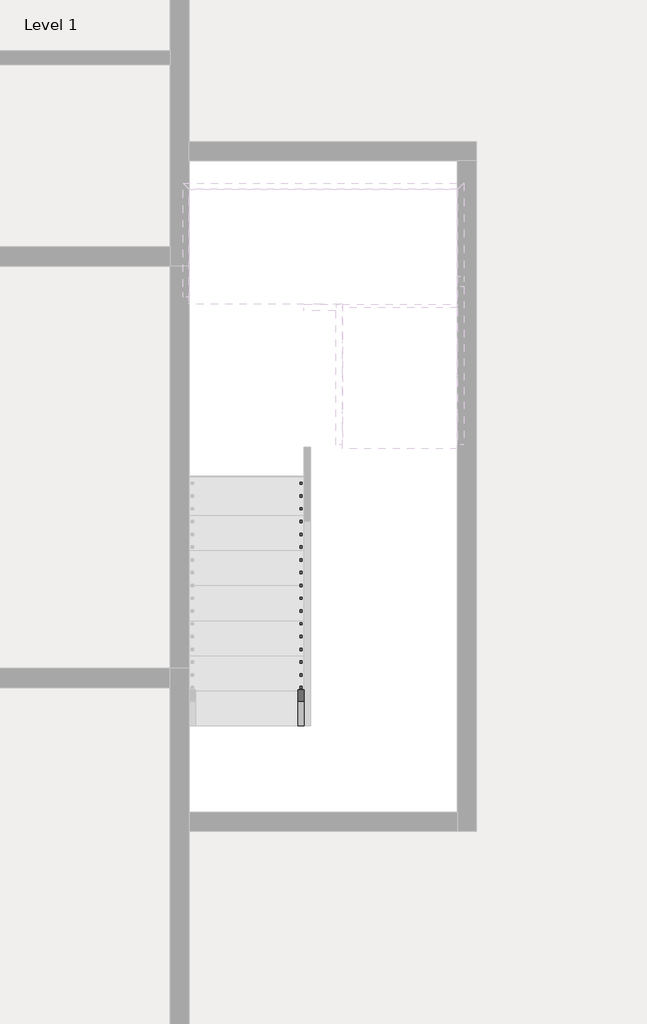
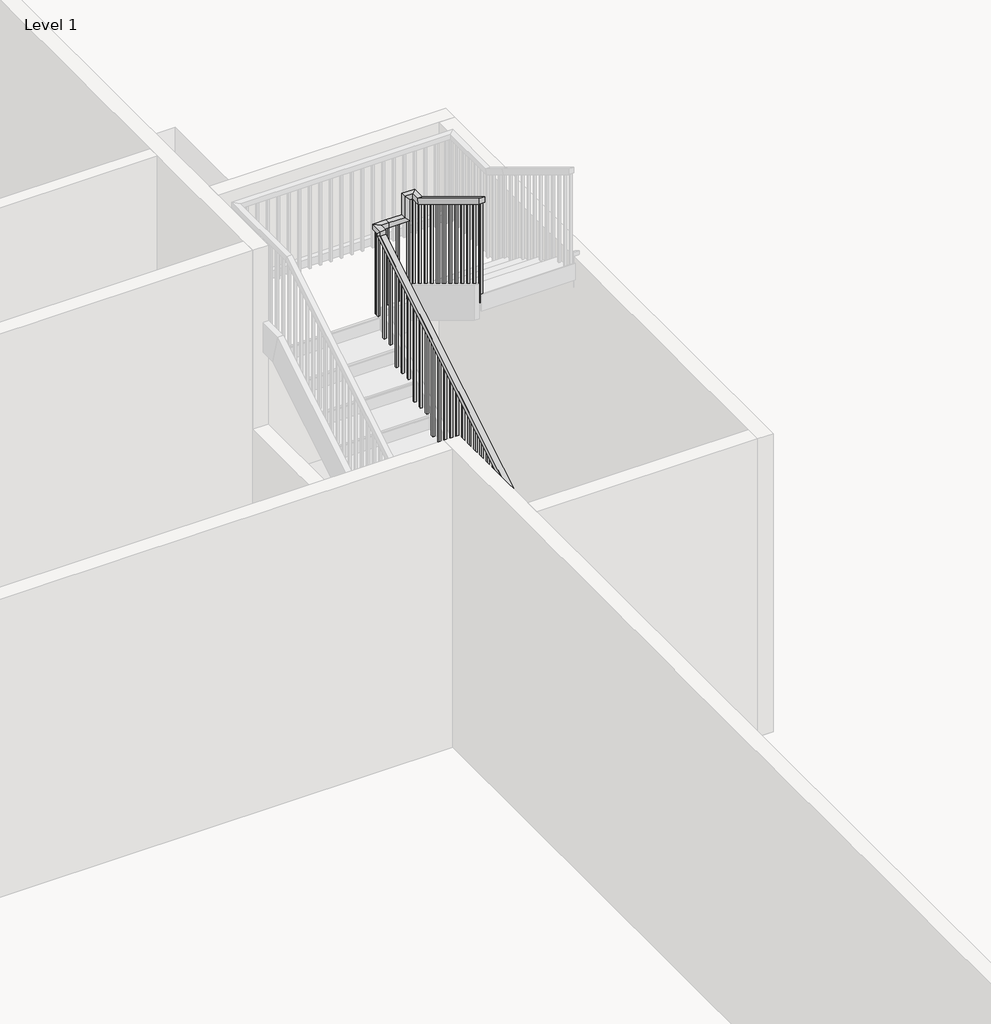
# One storey, part 7 of 8: 1 railing.
"""IFC4 building model written with IfcOpenShell, lengths in millimetres."""

from ifc_helpers import new_model, si_unit, frame, origin, place, context, project, spatial, polyline, outline, extrude, faceted_brep, element, save

model = new_model("IFC4")

# Units and contexts
model_context = context("Model", 3, world=origin())
ifc_project = project(units=[si_unit("LENGTHUNIT", "METRE", prefix="MILLI")], contexts=[model_context])

# Site, building, storey
site = spatial("IfcSite", under=ifc_project)
building = spatial("IfcBuilding", under=site)
storey = spatial("IfcBuildingStorey", under=building, Name="Level 1", Elevation=25234.6172466)

# Railing
placement = place(None, origin())
element("IfcRailing", 1, ObjectType="Handrail - Rectangular", at=placement, inside=storey, context=model_context, shape_type="SolidModel", body=[
    faceted_brep([(-2753.8415084, 19841.9216096, 26318.3505799), (-2753.8415084, 19841.9216096, 26258.9491197), (-2703.0415084, 19841.9216096, 26258.9491197), (-2703.0415084, 19841.9216096, 26318.3505799), (-2753.8415084, 23118.5216096, 28304.1687618), (-2753.8415084, 23169.3216096, 28275.5551803), (-2703.0415084, 23169.3216096, 28275.5551803), (-2703.0415084, 23118.5216096, 28304.1687618), (-2753.8415084, 23118.5216096, 28350.3505799), (-2753.8415084, 23169.3216096, 28299.5505799), (-2703.0415084, 23169.3216096, 28299.5505799), (-2703.0415084, 23118.5216096, 28350.3505799), (-2753.8415084, 23245.5216096, 28350.3505799), (-2753.8415084, 23245.5216096, 28299.5505799), (-2703.0415084, 23194.7216096, 28299.5505799), (-2703.0415084, 23194.7216096, 28350.3505799), (-2626.8415084, 23245.5216096, 28350.3505799), (-2626.8415084, 23245.5216096, 28299.5505799), (-2626.8415084, 23194.7216096, 28299.5505799), (-2626.8415084, 23194.7216096, 28350.3505799), (-2474.4415084, 23245.5216096, 28350.3505799), (-2423.6415084, 23245.5216096, 28299.5505799), (-2423.6415084, 23194.7216096, 28299.5505799), (-2474.4415084, 23194.7216096, 28350.3505799), (-2474.4415084, 23245.5216096, 28565.8657314), (-2423.6415084, 23245.5216096, 28515.0657314), (-2423.6415084, 23194.7216096, 28515.0657314), (-2474.4415084, 23194.7216096, 28565.8657314), (-2347.4415084, 23245.5216096, 28565.8657314), (-2347.4415084, 23245.5216096, 28515.0657314), (-2398.2415084, 23194.7216096, 28515.0657314), (-2398.2415084, 23194.7216096, 28565.8657314), (-2347.4415084, 23118.5216096, 28565.8657314), (-2347.4415084, 23104.3292002, 28515.0657314), (-2398.2415084, 23104.3292002, 28515.0657314), (-2398.2415084, 23118.5216096, 28565.8657314), (-2347.4415084, 22077.1216096, 29197.0172466), (-2398.2415084, 22077.1216096, 29197.0172466), (-2398.2415084, 22077.1216096, 29137.6157863), (-2347.4415084, 22077.1216096, 29137.6157863)], [[[0, 1, 2, 3]], [[1, 0, 4, 5]], [[2, 1, 5, 6]], [[3, 2, 6, 7]], [[0, 3, 7, 4]], [[5, 4, 8, 9]], [[6, 5, 9, 10]], [[7, 6, 10, 11]], [[4, 7, 11, 8]], [[9, 8, 12, 13]], [[10, 9, 13, 14]], [[11, 10, 14, 15]], [[8, 11, 15, 12]], [[13, 12, 16, 17]], [[14, 13, 17, 18]], [[15, 14, 18, 19]], [[12, 15, 19, 16]], [[17, 16, 20, 21]], [[18, 17, 21, 22]], [[19, 18, 22, 23]], [[16, 19, 23, 20]], [[21, 20, 24, 25]], [[22, 21, 25, 26]], [[23, 22, 26, 27]], [[20, 23, 27, 24]], [[25, 24, 28, 29]], [[26, 25, 29, 30]], [[27, 26, 30, 31]], [[24, 27, 31, 28]], [[29, 28, 32, 33]], [[30, 29, 33, 34]], [[31, 30, 34, 35]], [[28, 31, 35, 32]], [[36, 37, 38, 39]], [[33, 32, 36, 39]], [[34, 33, 39, 38]], [[35, 34, 38, 37]], [[32, 35, 37, 36]]]),
    extrude(outline(polyline([(22092.9966096, 29127.9945742), (22112.0466096, 29116.4491197), (22112.0466096, 28113.2839133), (22092.9966096, 28113.2839133), (22092.9966096, 29127.9945742)])), frame((-2382.3665084, 0.0, 0.0), z_axis=(1.0, 0.0, 0.0), x_axis=(0.0, 1.0, 0.0)), (0.0, 0.0, 1.0), 19.05),
    extrude(outline(polyline([(22194.5966096, 29066.4188167), (22213.6466096, 29054.8733621), (22213.6466096, 28113.2839133), (22194.5966096, 28113.2839133), (22194.5966096, 29066.4188167)])), frame((-2382.3665084, 0.0, 0.0), z_axis=(1.0, 0.0, 0.0), x_axis=(0.0, 1.0, 0.0)), (0.0, 0.0, 1.0), 19.05),
    extrude(outline(polyline([(22296.1966096, 29004.8430591), (22315.2466096, 28993.2976045), (22315.2466096, 28113.2839133), (22296.1966096, 28113.2839133), (22296.1966096, 29004.8430591)])), frame((-2382.3665084, 0.0, 0.0), z_axis=(1.0, 0.0, 0.0), x_axis=(0.0, 1.0, 0.0)), (0.0, 0.0, 1.0), 19.05),
    extrude(outline(polyline([(22397.7966096, 28943.2673015), (22416.8466096, 28931.721847), (22416.8466096, 27943.9505799), (22397.7966096, 27943.9505799), (22397.7966096, 28943.2673015)])), frame((-2382.3665084, 0.0, 0.0), z_axis=(1.0, 0.0, 0.0), x_axis=(0.0, 1.0, 0.0)), (0.0, 0.0, 1.0), 19.05),
    extrude(outline(polyline([(22499.3966096, 28881.6915439), (22518.4466096, 28870.1460894), (22518.4466096, 27943.9505799), (22499.3966096, 27943.9505799), (22499.3966096, 28881.6915439)])), frame((-2382.3665084, 0.0, 0.0), z_axis=(1.0, 0.0, 0.0), x_axis=(0.0, 1.0, 0.0)), (0.0, 0.0, 1.0), 19.05),
    extrude(outline(polyline([(22600.9966096, 28820.1157863), (22620.0466096, 28808.5703318), (22620.0466096, 27943.9505799), (22600.9966096, 27943.9505799), (22600.9966096, 28820.1157863)])), frame((-2382.3665084, 0.0, 0.0), z_axis=(1.0, 0.0, 0.0), x_axis=(0.0, 1.0, 0.0)), (0.0, 0.0, 1.0), 19.05),
    extrude(outline(polyline([(22702.5966096, 28758.5400288), (22721.6466096, 28746.9945742), (22721.6466096, 27774.6172466), (22702.5966096, 27774.6172466), (22702.5966096, 28758.5400288)])), frame((-2382.3665084, 0.0, 0.0), z_axis=(1.0, 0.0, 0.0), x_axis=(0.0, 1.0, 0.0)), (0.0, 0.0, 1.0), 19.05),
    extrude(outline(polyline([(22804.1966096, 28696.9642712), (22823.2466096, 28685.4188167), (22823.2466096, 27774.6172466), (22804.1966096, 27774.6172466), (22804.1966096, 28696.9642712)])), frame((-2382.3665084, 0.0, 0.0), z_axis=(1.0, 0.0, 0.0), x_axis=(0.0, 1.0, 0.0)), (0.0, 0.0, 1.0), 19.05),
    extrude(outline(polyline([(22905.7966096, 28635.3885136), (22924.8466096, 28623.8430591), (22924.8466096, 27774.6172466), (22905.7966096, 27774.6172466), (22905.7966096, 28635.3885136)])), frame((-2382.3665084, 0.0, 0.0), z_axis=(1.0, 0.0, 0.0), x_axis=(0.0, 1.0, 0.0)), (0.0, 0.0, 1.0), 19.05),
    extrude(outline(polyline([(23007.3966096, 28573.812756), (23026.4466096, 28562.2673015), (23026.4466096, 27605.2839133), (23007.3966096, 27605.2839133), (23007.3966096, 28573.812756)])), frame((-2382.3665084, 0.0, 0.0), z_axis=(1.0, 0.0, 0.0), x_axis=(0.0, 1.0, 0.0)), (0.0, 0.0, 1.0), 19.05),
    extrude(outline(polyline([(23108.9966096, 28512.2369985), (23128.0466096, 28500.6915439), (23128.0466096, 27605.2839133), (23108.9966096, 27605.2839133), (23108.9966096, 28512.2369985)])), frame((-2382.3665084, 0.0, 0.0), z_axis=(1.0, 0.0, 0.0), x_axis=(0.0, 1.0, 0.0)), (0.0, 0.0, 1.0), 19.05),
    extrude(outline(polyline([(-2433.1665084, 23210.5966096), (-2433.1665084, 23229.6466096), (-2414.1165084, 23229.6466096), (-2414.1165084, 23210.5966096), (-2433.1665084, 23210.5966096)])), frame((0.0, 0.0, 27435.9505799), z_axis=(0.0, 0.0, 1.0), x_axis=(1.0, 0.0, 0.0)), (0.0, 0.0, 1.0), 1079.1151515),
    extrude(outline(polyline([(-2534.7665084, 23210.5966096), (-2534.7665084, 23229.6466096), (-2515.7165084, 23229.6466096), (-2515.7165084, 23210.5966096), (-2534.7665084, 23210.5966096)])), frame((0.0, 0.0, 27435.9505799), z_axis=(0.0, 0.0, 1.0), x_axis=(1.0, 0.0, 0.0)), (0.0, 0.0, 1.0), 863.6),
    extrude(outline(polyline([(-2636.3665084, 23210.5966096), (-2636.3665084, 23229.6466096), (-2617.3165084, 23229.6466096), (-2617.3165084, 23210.5966096), (-2636.3665084, 23210.5966096)])), frame((0.0, 0.0, 27435.9505799), z_axis=(0.0, 0.0, 1.0), x_axis=(1.0, 0.0, 0.0)), (0.0, 0.0, 1.0), 863.6),
    extrude(outline(polyline([(-2718.9165084, 23185.1966096), (-2737.9665084, 23185.1966096), (-2737.9665084, 23204.2466096), (-2718.9165084, 23204.2466096), (-2718.9165084, 23185.1966096)])), frame((0.0, 0.0, 27435.9505799), z_axis=(0.0, 0.0, 1.0), x_axis=(1.0, 0.0, 0.0)), (0.0, 0.0, 1.0), 863.6),
    extrude(outline(polyline([(23083.5966096, 28223.6006348), (23102.6466096, 28235.1460894), (23102.6466096, 27266.6172466), (23083.5966096, 27266.6172466), (23083.5966096, 28223.6006348)])), frame((-2737.9665084, 0.0, 0.0), z_axis=(1.0, 0.0, 0.0), x_axis=(0.0, 1.0, 0.0)), (0.0, 0.0, 1.0), 19.05),
    extrude(outline(polyline([(22981.9966096, 28162.0248773), (23001.0466096, 28173.5703318), (23001.0466096, 27266.6172466), (22981.9966096, 27266.6172466), (22981.9966096, 28162.0248773)])), frame((-2737.9665084, 0.0, 0.0), z_axis=(1.0, 0.0, 0.0), x_axis=(0.0, 1.0, 0.0)), (0.0, 0.0, 1.0), 19.05),
    extrude(outline(polyline([(22880.3966096, 28100.4491197), (22899.4466096, 28111.9945742), (22899.4466096, 27097.2839133), (22880.3966096, 27097.2839133), (22880.3966096, 28100.4491197)])), frame((-2737.9665084, 0.0, 0.0), z_axis=(1.0, 0.0, 0.0), x_axis=(0.0, 1.0, 0.0)), (0.0, 0.0, 1.0), 19.05),
    extrude(outline(polyline([(22778.7966096, 28038.8733621), (22797.8466096, 28050.4188167), (22797.8466096, 27097.2839133), (22778.7966096, 27097.2839133), (22778.7966096, 28038.8733621)])), frame((-2737.9665084, 0.0, 0.0), z_axis=(1.0, 0.0, 0.0), x_axis=(0.0, 1.0, 0.0)), (0.0, 0.0, 1.0), 19.05),
    extrude(outline(polyline([(22677.1966096, 27977.2976045), (22696.2466096, 27988.8430591), (22696.2466096, 27097.2839133), (22677.1966096, 27097.2839133), (22677.1966096, 27977.2976045)])), frame((-2737.9665084, 0.0, 0.0), z_axis=(1.0, 0.0, 0.0), x_axis=(0.0, 1.0, 0.0)), (0.0, 0.0, 1.0), 19.05),
    extrude(outline(polyline([(22575.5966096, 27915.721847), (22594.6466096, 27927.2673015), (22594.6466096, 26927.9505799), (22575.5966096, 26927.9505799), (22575.5966096, 27915.721847)])), frame((-2737.9665084, 0.0, 0.0), z_axis=(1.0, 0.0, 0.0), x_axis=(0.0, 1.0, 0.0)), (0.0, 0.0, 1.0), 19.05),
    extrude(outline(polyline([(22473.9966096, 27854.1460894), (22493.0466096, 27865.6915439), (22493.0466096, 26927.9505799), (22473.9966096, 26927.9505799), (22473.9966096, 27854.1460894)])), frame((-2737.9665084, 0.0, 0.0), z_axis=(1.0, 0.0, 0.0), x_axis=(0.0, 1.0, 0.0)), (0.0, 0.0, 1.0), 19.05),
    extrude(outline(polyline([(22372.3966096, 27792.5703318), (22391.4466096, 27804.1157863), (22391.4466096, 26927.9505799), (22372.3966096, 26927.9505799), (22372.3966096, 27792.5703318)])), frame((-2737.9665084, 0.0, 0.0), z_axis=(1.0, 0.0, 0.0), x_axis=(0.0, 1.0, 0.0)), (0.0, 0.0, 1.0), 19.05),
    extrude(outline(polyline([(22270.7966096, 27730.9945742), (22289.8466096, 27742.5400288), (22289.8466096, 26758.6172466), (22270.7966096, 26758.6172466), (22270.7966096, 27730.9945742)])), frame((-2737.9665084, 0.0, 0.0), z_axis=(1.0, 0.0, 0.0), x_axis=(0.0, 1.0, 0.0)), (0.0, 0.0, 1.0), 19.05),
    extrude(outline(polyline([(22169.1966096, 27669.4188167), (22188.2466096, 27680.9642712), (22188.2466096, 26758.6172466), (22169.1966096, 26758.6172466), (22169.1966096, 27669.4188167)])), frame((-2737.9665084, 0.0, 0.0), z_axis=(1.0, 0.0, 0.0), x_axis=(0.0, 1.0, 0.0)), (0.0, 0.0, 1.0), 19.05),
    extrude(outline(polyline([(22067.5966096, 27607.8430591), (22086.6466096, 27619.3885136), (22086.6466096, 26758.6172466), (22067.5966096, 26758.6172466), (22067.5966096, 27607.8430591)])), frame((-2737.9665084, 0.0, 0.0), z_axis=(1.0, 0.0, 0.0), x_axis=(0.0, 1.0, 0.0)), (0.0, 0.0, 1.0), 19.05),
    extrude(outline(polyline([(21965.9966096, 27546.2673015), (21985.0466096, 27557.812756), (21985.0466096, 26589.2839133), (21965.9966096, 26589.2839133), (21965.9966096, 27546.2673015)])), frame((-2737.9665084, 0.0, 0.0), z_axis=(1.0, 0.0, 0.0), x_axis=(0.0, 1.0, 0.0)), (0.0, 0.0, 1.0), 19.05),
    extrude(outline(polyline([(21864.3966096, 27484.6915439), (21883.4466096, 27496.2369985), (21883.4466096, 26589.2839133), (21864.3966096, 26589.2839133), (21864.3966096, 27484.6915439)])), frame((-2737.9665084, 0.0, 0.0), z_axis=(1.0, 0.0, 0.0), x_axis=(0.0, 1.0, 0.0)), (0.0, 0.0, 1.0), 19.05),
    extrude(outline(polyline([(21762.7966096, 27423.1157863), (21781.8466096, 27434.6612409), (21781.8466096, 26419.9505799), (21762.7966096, 26419.9505799), (21762.7966096, 27423.1157863)])), frame((-2737.9665084, 0.0, 0.0), z_axis=(1.0, 0.0, 0.0), x_axis=(0.0, 1.0, 0.0)), (0.0, 0.0, 1.0), 19.05),
    extrude(outline(polyline([(21661.1966096, 27361.5400288), (21680.2466096, 27373.0854833), (21680.2466096, 26419.9505799), (21661.1966096, 26419.9505799), (21661.1966096, 27361.5400288)])), frame((-2737.9665084, 0.0, 0.0), z_axis=(1.0, 0.0, 0.0), x_axis=(0.0, 1.0, 0.0)), (0.0, 0.0, 1.0), 19.05),
    extrude(outline(polyline([(21559.5966096, 27299.9642712), (21578.6466096, 27311.5097257), (21578.6466096, 26419.9505799), (21559.5966096, 26419.9505799), (21559.5966096, 27299.9642712)])), frame((-2737.9665084, 0.0, 0.0), z_axis=(1.0, 0.0, 0.0), x_axis=(0.0, 1.0, 0.0)), (0.0, 0.0, 1.0), 19.05),
    extrude(outline(polyline([(21457.9966096, 27238.3885136), (21477.0466096, 27249.9339682), (21477.0466096, 26250.6172466), (21457.9966096, 26250.6172466), (21457.9966096, 27238.3885136)])), frame((-2737.9665084, 0.0, 0.0), z_axis=(1.0, 0.0, 0.0), x_axis=(0.0, 1.0, 0.0)), (0.0, 0.0, 1.0), 19.05),
    extrude(outline(polyline([(21356.3966096, 27176.812756), (21375.4466096, 27188.3582106), (21375.4466096, 26250.6172466), (21356.3966096, 26250.6172466), (21356.3966096, 27176.812756)])), frame((-2737.9665084, 0.0, 0.0), z_axis=(1.0, 0.0, 0.0), x_axis=(0.0, 1.0, 0.0)), (0.0, 0.0, 1.0), 19.05),
    extrude(outline(polyline([(21254.7966096, 27115.2369985), (21273.8466096, 27126.782453), (21273.8466096, 26250.6172466), (21254.7966096, 26250.6172466), (21254.7966096, 27115.2369985)])), frame((-2737.9665084, 0.0, 0.0), z_axis=(1.0, 0.0, 0.0), x_axis=(0.0, 1.0, 0.0)), (0.0, 0.0, 1.0), 19.05),
    extrude(outline(polyline([(21153.1966096, 27053.6612409), (21172.2466096, 27065.2066954), (21172.2466096, 26081.2839133), (21153.1966096, 26081.2839133), (21153.1966096, 27053.6612409)])), frame((-2737.9665084, 0.0, 0.0), z_axis=(1.0, 0.0, 0.0), x_axis=(0.0, 1.0, 0.0)), (0.0, 0.0, 1.0), 19.05),
    extrude(outline(polyline([(21051.5966096, 26992.0854833), (21070.6466096, 27003.6309379), (21070.6466096, 26081.2839133), (21051.5966096, 26081.2839133), (21051.5966096, 26992.0854833)])), frame((-2737.9665084, 0.0, 0.0), z_axis=(1.0, 0.0, 0.0), x_axis=(0.0, 1.0, 0.0)), (0.0, 0.0, 1.0), 19.05),
    extrude(outline(polyline([(20949.9966096, 26930.5097257), (20969.0466096, 26942.0551803), (20969.0466096, 26081.2839133), (20949.9966096, 26081.2839133), (20949.9966096, 26930.5097257)])), frame((-2737.9665084, 0.0, 0.0), z_axis=(1.0, 0.0, 0.0), x_axis=(0.0, 1.0, 0.0)), (0.0, 0.0, 1.0), 19.05),
    extrude(outline(polyline([(20848.3966096, 26868.9339682), (20867.4466096, 26880.4794227), (20867.4466096, 25911.9505799), (20848.3966096, 25911.9505799), (20848.3966096, 26868.9339682)])), frame((-2737.9665084, 0.0, 0.0), z_axis=(1.0, 0.0, 0.0), x_axis=(0.0, 1.0, 0.0)), (0.0, 0.0, 1.0), 19.05),
    extrude(outline(polyline([(20746.7966096, 26807.3582106), (20765.8466096, 26818.9036651), (20765.8466096, 25911.9505799), (20746.7966096, 25911.9505799), (20746.7966096, 26807.3582106)])), frame((-2737.9665084, 0.0, 0.0), z_axis=(1.0, 0.0, 0.0), x_axis=(0.0, 1.0, 0.0)), (0.0, 0.0, 1.0), 19.05),
    extrude(outline(polyline([(20645.1966096, 26745.782453), (20664.2466096, 26757.3279076), (20664.2466096, 25742.6172466), (20645.1966096, 25742.6172466), (20645.1966096, 26745.782453)])), frame((-2737.9665084, 0.0, 0.0), z_axis=(1.0, 0.0, 0.0), x_axis=(0.0, 1.0, 0.0)), (0.0, 0.0, 1.0), 19.05),
    extrude(outline(polyline([(20543.5966096, 26684.2066954), (20562.6466096, 26695.75215), (20562.6466096, 25742.6172466), (20543.5966096, 25742.6172466), (20543.5966096, 26684.2066954)])), frame((-2737.9665084, 0.0, 0.0), z_axis=(1.0, 0.0, 0.0), x_axis=(0.0, 1.0, 0.0)), (0.0, 0.0, 1.0), 19.05),
    extrude(outline(polyline([(20441.9966096, 26622.6309379), (20461.0466096, 26634.1763924), (20461.0466096, 25742.6172466), (20441.9966096, 25742.6172466), (20441.9966096, 26622.6309379)])), frame((-2737.9665084, 0.0, 0.0), z_axis=(1.0, 0.0, 0.0), x_axis=(0.0, 1.0, 0.0)), (0.0, 0.0, 1.0), 19.05),
    extrude(outline(polyline([(20340.3966096, 26561.0551803), (20359.4466096, 26572.6006348), (20359.4466096, 25573.2839133), (20340.3966096, 25573.2839133), (20340.3966096, 26561.0551803)])), frame((-2737.9665084, 0.0, 0.0), z_axis=(1.0, 0.0, 0.0), x_axis=(0.0, 1.0, 0.0)), (0.0, 0.0, 1.0), 19.05),
    extrude(outline(polyline([(20238.7966096, 26499.4794227), (20257.8466096, 26511.0248773), (20257.8466096, 25573.2839133), (20238.7966096, 25573.2839133), (20238.7966096, 26499.4794227)])), frame((-2737.9665084, 0.0, 0.0), z_axis=(1.0, 0.0, 0.0), x_axis=(0.0, 1.0, 0.0)), (0.0, 0.0, 1.0), 19.05),
    extrude(outline(polyline([(20137.1966096, 26437.9036651), (20156.2466096, 26449.4491197), (20156.2466096, 25573.2839133), (20137.1966096, 25573.2839133), (20137.1966096, 26437.9036651)])), frame((-2737.9665084, 0.0, 0.0), z_axis=(1.0, 0.0, 0.0), x_axis=(0.0, 1.0, 0.0)), (0.0, 0.0, 1.0), 19.05),
    extrude(outline(polyline([(20035.5966096, 26376.3279076), (20054.6466096, 26387.8733621), (20054.6466096, 25403.9505799), (20035.5966096, 25403.9505799), (20035.5966096, 26376.3279076)])), frame((-2737.9665084, 0.0, 0.0), z_axis=(1.0, 0.0, 0.0), x_axis=(0.0, 1.0, 0.0)), (0.0, 0.0, 1.0), 19.05),
    extrude(outline(polyline([(19933.9966096, 26314.75215), (19953.0466096, 26326.2976045), (19953.0466096, 25403.9505799), (19933.9966096, 25403.9505799), (19933.9966096, 26314.75215)])), frame((-2737.9665084, 0.0, 0.0), z_axis=(1.0, 0.0, 0.0), x_axis=(0.0, 1.0, 0.0)), (0.0, 0.0, 1.0), 19.05),
    extrude(outline(polyline([(-2382.3665084, 23210.5966096), (-2382.3665084, 23229.6466096), (-2363.3165084, 23229.6466096), (-2363.3165084, 23210.5966096), (-2382.3665084, 23210.5966096)])), frame((0.0, 0.0, 27435.9505799), z_axis=(0.0, 0.0, 1.0), x_axis=(1.0, 0.0, 0.0)), (0.0, 0.0, 1.0), 1079.1151515),
    extrude(outline(polyline([(-2718.9165084, 23210.5966096), (-2737.9665084, 23210.5966096), (-2737.9665084, 23229.6466096), (-2718.9165084, 23229.6466096), (-2718.9165084, 23210.5966096)])), frame((0.0, 0.0, 27435.9505799), z_axis=(0.0, 0.0, 1.0), x_axis=(1.0, 0.0, 0.0)), (0.0, 0.0, 1.0), 863.6),
    extrude(outline(polyline([(22077.1216096, 29137.6157863), (22096.1716096, 29126.0703318), (22096.1716096, 28113.2839133), (22077.1216096, 28113.2839133), (22077.1216096, 29137.6157863)])), frame((-2382.3665084, 0.0, 0.0), z_axis=(1.0, 0.0, 0.0), x_axis=(0.0, 1.0, 0.0)), (0.0, 0.0, 1.0), 19.05),
    extrude(outline(polyline([(19841.9216096, 26258.9491197), (19860.9716096, 26270.4945742), (19860.9716096, 25403.9505799), (19841.9216096, 25403.9505799), (19841.9216096, 26258.9491197)])), frame((-2737.9665084, 0.0, 0.0), z_axis=(1.0, 0.0, 0.0), x_axis=(0.0, 1.0, 0.0)), (0.0, 0.0, 1.0), 19.05),
])

save(model, "model.ifc")

# Revit data of these elements
# Type "Handrail - Rectangular"
#   Assembly Code = "C2010400"
#   built-in parameter 1008612 = 0.0416667 (stored number, unit not read)
#   built-in parameter 1008611 = 0.0416667 (stored number, unit not read)
#   built-in parameter 1008609 = 0.333333 (stored number, unit not read)
#   built-in parameter 1008604 = 0.166667 (stored number, unit not read)
#   built-in parameter 1008603 = 0.166667 (stored number, unit not read)
#   Railing Height = 3' - 0"
#   built-in parameter 1008630 = 2
#   built-in parameter 1008610 = 2
#   built-in parameter 1008618 = Baluster - Square : 3/4"
# Element 1 (IfcRailing, "Handrail - Rectangular")
#   Phase Created = New Construction
